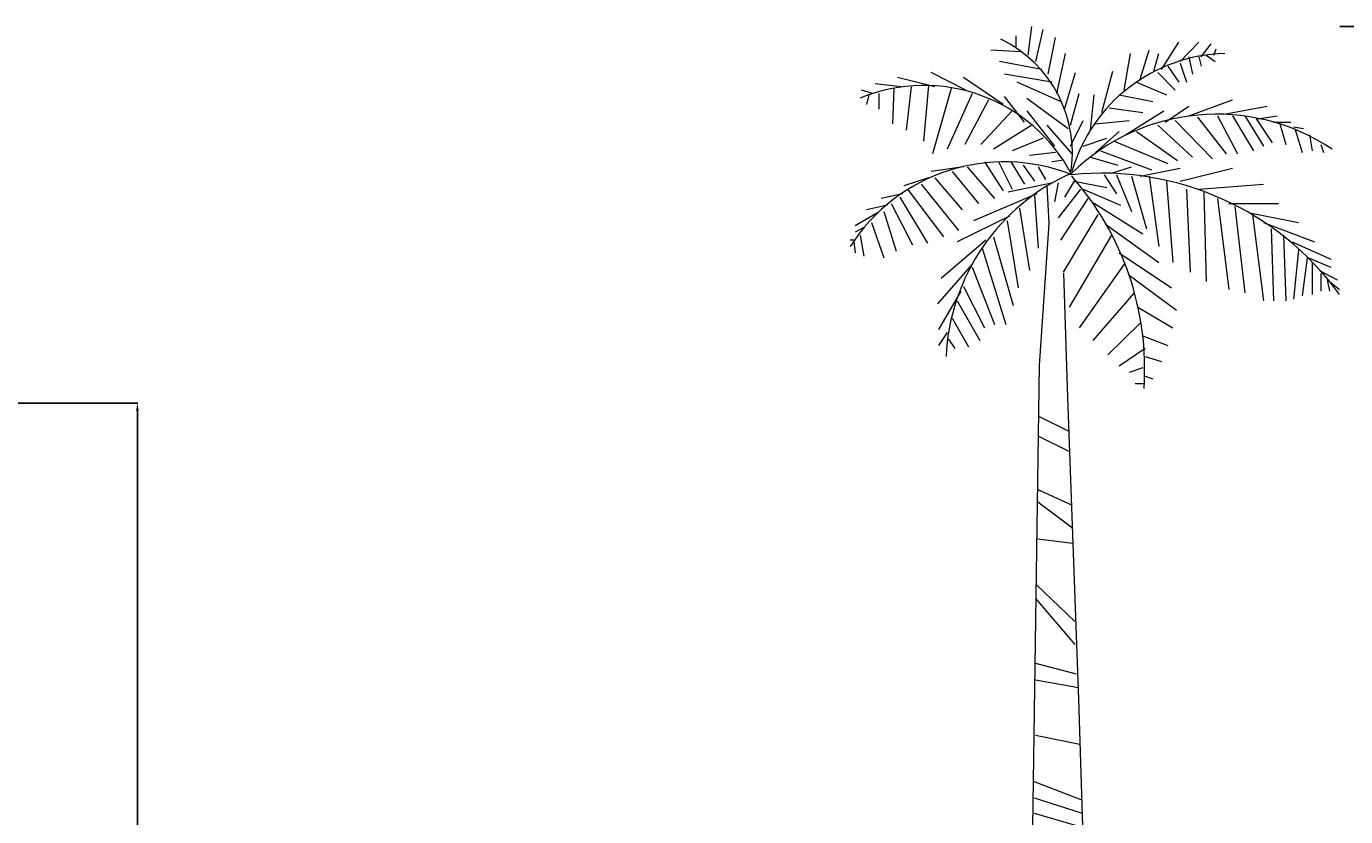
# Model space of a CAD drawing. Units: inches. Extents: x 481 to 2783, y 1975 to 3327.
# Tile 3 of 13: x 910 to 1326, y 2282 to 2531. Entities that reach past the tile are written whole.
import ezdxf

# ---------------------------------------------------------------- set-up
doc = ezdxf.new("R2010")
doc.units = ezdxf.units.IN
doc.header["$MEASUREMENT"] = 0
doc.layers.add('A-ANNO-DIMS', color=50, linetype='Continuous', lineweight=18)
doc.layers.add('L-PLNT', color=7, linetype='Continuous', lineweight=13)
doc.styles.get("Standard").update_dxf_attribs({"font": 'arial.ttf'})
doc.dimstyles.get("Standard").update_dxf_attribs({"dimtxt": 2.5, "dimasz": 2.5, "dimexe": 0.18, "dimexo": 0.0625, "dimgap": 0.09, "dimtad": 0, "dimtih": 1, "dimtoh": 1, "dimzin": 0, "dimdsep": 46, "dimlunit": 3, "dimtxsty": 'Standard', "dimcen": 0.09, "dimadec": 0, "dimazin": 0, "dimtfac": 1, "dimtofl": 0, "dimtmove": 0, "dimatfit": 3, "dimfxl": 1, "dimtolj": 1, "dimtzin": 0, "dimarcsym": 0})

# ---------------------------------------------------------------- blocks, each defined once
blk = doc.blocks.new('Tree - palm elevation')
for p, q in [((-5.567, 196.707), (-4.987, 201.167)), ((-7.5, 199.68), (-7.5, 197.946)), ((-4.407, 195.716), (-3.247, 200.672)), ((-2.474, 193.733), (-1.315, 199.433)), ((15.116, 194.477), (17.822, 198.689)), ((18.015, 195.716), (20.914, 198.689)), ((-6.727, 197.202), (-11.366, 197.45)), ((-1.121, 190.759), (0.232, 196.955)), ((9.317, 191.255), (10.283, 196.955)), ((11.829, 192.99), (13.182, 197.45)), ((13.956, 194.229), (14.729, 196.955)), ((21.301, 196.459), (22.847, 198.441)), ((22.074, 196.707), (23.427, 195.716)), ((23.234, 196.707), (23.62, 197.698)), ((-3.441, 194.477), (-10.013, 195.716)), ((16.082, 194.972), (17.822, 192.494)), ((18.015, 195.468), (18.981, 192.494)), ((19.368, 196.459), (19.948, 193.733)), ((20.914, 196.459), (21.301, 194.972)), ((-20.064, 191.751), (-25.863, 193.238)), ((-15.232, 191.255), (-20.644, 193.981)), ((-9.433, 189.025), (-15.618, 193.238)), ((-1.894, 192.494), (-9.24, 193.733)), ((0.038, 188.281), (1.778, 193.981)), ((5.837, 187.786), (7.577, 194.229)), ((14.536, 193.981), (17.242, 191.255)), ((-29.729, 190.759), (-31.469, 191.255)), ((-30.309, 190.512), (-30.695, 189.025)), ((-25.283, 191.751), (-29.342, 192.246)), ((-28.763, 190.759), (-28.763, 188.281)), ((-26.443, 191.503), (-26.636, 186.051)), ((-23.737, 191.751), (-24.51, 185.06)), ((-21.031, 191.998), (-21.804, 183.325)), ((-17.551, 191.503), (-20.451, 181.343)), ((-14.265, 190.759), (-18.131, 182.086)), ((-0.541, 189.52), (-7.307, 192.494)), ((1.005, 185.803), (2.358, 190.759)), ((4.098, 185.06), (4.678, 190.512)), ((8.544, 190.512), (13.763, 189.52)), ((11.25, 192.494), (15.889, 190.512)), ((-11.753, 189.768), (-15.425, 182.83)), ((-6.147, 186.299), (-9.24, 190.264)), ((-5.76, 190.016), (0.618, 185.308)), ((6.997, 188.529), (12.216, 187.786)), ((15.695, 186.299), (19.368, 188.777)), ((19.368, 187.29), (26.133, 189.768)), ((24.78, 187.538), (31.546, 188.777)), ((-8.08, 188.034), (-12.912, 182.83)), ((-5.76, 188.034), (-1.508, 182.582)), ((1.005, 182.582), (2.938, 186.547)), ((4.871, 186.051), (10.09, 186.547)), ((9.51, 184.317), (15.502, 188.034)), ((17.242, 186.547), (23.041, 180.599)), ((20.721, 187.042), (25.167, 181.343)), ((23.814, 187.29), (26.907, 181.343)), ((26.133, 187.29), (29.419, 181.838)), ((28.066, 187.29), (30.966, 182.582)), ((29.806, 186.795), (32.319, 183.078)), ((29.999, 186.795), (33.092, 187.29)), ((-4.987, 185.803), (-10.979, 182.086)), ((-2.668, 185.803), (1.198, 181.343)), ((4.871, 181.591), (8.544, 184.812)), ((11.25, 184.812), (17.628, 180.352)), ((14.536, 185.803), (19.948, 180.847)), ((32.512, 186.299), (35.218, 186.299)), ((33.479, 186.051), (34.445, 182.83)), ((35.605, 185.556), (37.151, 185.308)), ((35.798, 185.308), (36.958, 181.591)), ((38.118, 184.317), (38.504, 181.838)), ((-3.247, 183.821), (-8.08, 181.838)), ((2.938, 182.582), (6.61, 183.821)), ((7.77, 183.325), (16.082, 179.856)), ((39.857, 182.83), (40.244, 181.591)), ((-1.315, 181.591), (-5.374, 181.095)), ((-0.348, 180.352), (-1.894, 180.104)), ((4.098, 180.847), (8.35, 179.608)), ((5.644, 181.838), (13.569, 178.865)), ((-15.618, 179.36), (-20.644, 178.617)), ((-17.358, 178.617), (-13.299, 173.661)), ((-15.038, 179.36), (-10.786, 174.404)), ((-12.332, 180.104), (-9.433, 175.643)), ((-10.206, 180.104), (-8.08, 175.891)), ((-8.273, 180.104), (-6.147, 176.635)), ((-6.34, 179.608), (-4.6, 177.13)), ((-4.021, 179.36), (-2.861, 177.378)), ((7.384, 178.369), (10.476, 179.36)), ((11.829, 177.874), (18.015, 179.113)), ((18.015, 177.13), (26.133, 179.113)), ((-21.031, 177.626), (-24.897, 176.387)), ((-22.191, 176.635), (-16.391, 169.448)), ((-20.064, 177.626), (-15.812, 172.67)), ((-1.701, 176.882), (-8.66, 175.396)), ((-2.668, 176.387), (-2.376, 170.594)), ((-0.928, 176.882), (-1.508, 173.909)), ((1.585, 177.13), (0.038, 174.652)), ((1.585, 177.13), (6.61, 176.139)), ((6.224, 178.121), (8.157, 175.148)), ((8.157, 178.121), (10.476, 172.422)), ((10.476, 177.874), (12.796, 169.696)), ((13.182, 177.874), (14.729, 166.97)), ((15.889, 177.13), (16.855, 164.492)), ((20.914, 175.891), (30.966, 176.635)), ((-25.09, 175.148), (-28.376, 174.404)), ((-25.476, 174.652), (-21.224, 167.466)), ((-24.317, 175.891), (-18.711, 168.457)), ((-4.214, 175.148), (-14.072, 170.935)), ((-4.6, 174.9), (-4.021, 166.722)), ((2.551, 175.891), (-0.928, 171.431)), ((3.711, 174.404), (-0.541, 167.961)), ((2.938, 175.891), (8.737, 173.413)), ((18.981, 175.891), (19.561, 163.005)), ((21.688, 175.396), (22.074, 161.518)), ((23.814, 174.404), (25.554, 160.279)), ((-28.956, 172.174), (-32.435, 170.192)), ((-27.409, 173.413), (-30.695, 172.67)), ((-27.989, 172.422), (-26.056, 166.227)), ((-26.829, 173.661), (-23.544, 167.218)), ((-6.92, 172.917), (-5.374, 163.253)), ((4.291, 173.909), (12.216, 168.953)), ((25.554, 173.661), (33.285, 173.661)), ((26.52, 173.165), (28.066, 159.784)), ((28.839, 172.174), (36.378, 170.687)), ((-29.922, 170.687), (-27.989, 165.235)), ((-8.466, 171.678), (-16.585, 167.713)), ((-8.853, 170.935), (-7.113, 160.527)), ((5.257, 171.926), (-0.155, 163.005)), ((6.417, 170.439), (14.729, 164.492)), ((29.226, 171.926), (30.966, 158.545)), ((30.966, 170.687), (38.891, 167.713)), ((-32.628, 167.961), (-33.208, 167.961)), ((-31.082, 169.944), (-32.435, 169.2)), ((-31.662, 168.705), (-31.082, 165.483)), ((-12.139, 167.961), (-19.098, 162.014)), ((-10.979, 168.457), (-7.887, 157.801)), ((7.384, 168.705), (0.812, 157.553)), ((32.126, 169.696), (32.512, 158.545)), ((34.058, 168.705), (34.445, 158.545)), ((-32.628, 167.713), (-32.435, 165.979)), ((-12.719, 166.722), (-9.046, 154.828)), ((8.544, 165.979), (16.662, 160.527)), ((35.412, 167.713), (41.404, 164.988)), ((36.378, 166.474), (35.605, 158.792)), ((-14.265, 164.244), (-19.678, 158.049)), ((9.317, 164.244), (2.358, 154.332)), ((37.731, 165.235), (36.958, 159.288)), ((37.924, 165.235), (41.404, 163.749)), ((38.504, 164.492), (38.504, 159.536)), ((-14.265, 163.749), (-10.786, 154.828)), ((10.09, 162.51), (17.435, 157.058)), ((39.664, 163.253), (42.37, 161.766)), ((39.857, 162.757), (39.857, 160.031)), ((-16.005, 160.031), (-19.484, 154.084)), ((-15.618, 160.775), (-12.332, 154.332)), ((10.863, 159.784), (4.484, 152.35)), ((40.824, 161.766), (41.21, 160.031)), ((41.21, 161.518), (42.757, 160.279)), ((-16.585, 158.545), (-13.106, 152.35)), ((-17.358, 155.819), (-14.845, 151.358)), ((11.443, 157.553), (16.855, 154.332)), ((11.829, 155.075), (6.804, 150.119)), ((-18.131, 153.589), (-19.484, 151.606)), ((-17.938, 152.597), (-16.972, 151.111)), ((12.216, 153.093), (16.082, 151.606)), ((12.603, 151.111), (8.544, 148.385)), ((12.603, 149.872), (15.116, 149.128)), ((12.216, 148.137), (10.09, 147.393)), ((12.409, 145.659), (11.056, 145.659)), ((12.409, 146.898), (13.763, 146.402)), ((-4.081, 140.645), (0.753, 138.261)), ((-4.081, 137.547), (0.753, 135.163)), ((-4.081, 129.205), (1.124, 126.821)), ((-4.081, 127.298), (1.31, 123.246)), ((-4.081, 121.578), (1.31, 120.863)), ((-4.267, 114.428), (1.682, 108.708)), ((-4.453, 112.283), (1.682, 105.133)), ((-4.639, 102.273), (1.868, 100.604)), ((-4.453, 99.651), (2.24, 98.459)), ((-4.453, 91.071), (2.426, 89.641)), ((-4.825, 83.921), (2.612, 81.061)), ((-4.639, 81.299), (2.797, 78.916)), ((-4.639, 78.916), (2.797, 76.771))]:
    blk.add_line(p, q)
for points in [[(-2.363, 170.553), (-3.88, 148.505), (-4.988, 69.634), (-3.325, 24.869), (0, 0)], [(-0.116, 162.848), (0.554, 143.532), (2.217, 96.635), (3.88, 44.054), (7.76, 12.079), (11.64, 0)]]:
    blk.add_lwpolyline(points)
for centre, radius, start, end in [((-18.427, 181.448), 19.715, 350.285, 64.11229), ((25.595, 171.567), 25.395, 91.40319, 163.882), ((-21.738, 166.094), 25.899, 27.67115, 112.5305), ((23.687, 155.341), 32.188, 56.19272, 134.3213), ((-9.259, 151.732), 28.386, 68.38311, 147.5322), ((14.394, 148.393), 32.752, 113.7592, 177.4133), ((5.828, 132.718), 45.639, 35.98777, 95.82273), ((-32.8, 147.923), 45.309, 356.1943, 41.37848)]:
    blk.add_arc(centre, radius, start, end)
blk = doc.blocks.new('*D54')
at = {"layer": 'A-ANNO-DIMS', "color": 0, "lineweight": -2, "transparency": 16777216}
for p, q in [((1324.1, 2531.22), (1385.48, 2531.22)), ((1385.3, 2528.72), (1385.3, 2328.4)), ((1385.3, 2125.32), (1385.3, 2325.64)), ((1324.1, 2122.82), (1385.48, 2122.82))]:
    blk.add_line(p, q, dxfattribs=at)
at = {"layer": 'A-ANNO-DIMS', "color": 0, "transparency": 16777216}
for points in [[(1384.88, 2528.72), (1385.72, 2528.72), (1385.3, 2531.22)], [(1384.88, 2125.32), (1385.72, 2125.32), (1385.3, 2122.82)]]:
    blk.add_solid(points, dxfattribs=at)
at = {"layer": 'Defpoints', "color": 0, "transparency": 16777216}
for p in [(1324.04, 2531.22), (1385.3, 2531.22), (1324.04, 2122.82)]:
    blk.add_point(p, dxfattribs=at)
at = {"layer": 'A-ANNO-DIMS', "color": 0, "transparency": 16777216, "insert": (1385.3, 2327.02), "char_height": 2.5, "attachment_point": 5}
blk.add_mtext('\\A1;PALM 34\'-0 1/2"', dxfattribs=at)
blk = doc.blocks.new('*D58')
at = {"layer": 'A-ANNO-DIMS', "color": 0, "lineweight": -2, "transparency": 16777216}
for p, q in [((901.81, 2412.41), (945.37, 2412.41)), ((945.19, 2409.91), (945.19, 2269)), ((945.19, 2125.32), (945.19, 2266.23)), ((901.81, 2122.82), (945.37, 2122.82))]:
    blk.add_line(p, q, dxfattribs=at)
at = {"layer": 'A-ANNO-DIMS', "color": 0, "transparency": 16777216}
for points in [[(944.77, 2409.91), (945.61, 2409.91), (945.19, 2412.41)], [(944.77, 2125.32), (945.61, 2125.32), (945.19, 2122.82)]]:
    blk.add_solid(points, dxfattribs=at)
at = {"layer": 'Defpoints', "color": 0, "transparency": 16777216}
for p in [(901.75, 2412.41), (945.19, 2412.41), (901.75, 2122.82)]:
    blk.add_point(p, dxfattribs=at)
at = {"layer": 'A-ANNO-DIMS', "color": 0, "transparency": 16777216, "insert": (945.19, 2267.62), "char_height": 2.5, "attachment_point": 5}
blk.add_mtext('\\A1;EVERGREEN 24\'-1 1/2"', dxfattribs=at)

msp = doc.modelspace()

# ---------------------------------------------------------------- block references
at = {"layer": 'L-PLNT', "xscale": 2.030135039985482, "yscale": 2.030135039985482, "zscale": 2.030135039985482}
msp.add_blockref('Tree - palm elevation', (1237.239, 2122.821), dxfattribs=at)

# ---------------------------------------------------------------- dimensions: what is measured, and where the dimension line sits
at = {"layer": 'A-ANNO-DIMS'}
for base, p1, p2, text, picture, middle in [((1385.301, 2531.217), (1324.042, 2122.821), (1324.042, 2531.217), 'PALM <>', '*D54', (1385.301, 2327.019)), ((945.19, 2412.413), (901.751, 2122.821), (901.751, 2412.413), 'EVERGREEN <>', '*D58', (945.19, 2267.617))]:
    dim = msp.add_linear_dim(base=base, p1=p1, p2=p2, angle=90, text=text, dimstyle='Standard', override={"dimdec": 1, "dimlfac": 1, "dimrnd": 0, "dimzin": 1, "dimdsep": 46, "dimlunit": 4, "dimfrac": 2}, dxfattribs=at)
    dim.commit()
    dim.dimension.update_dxf_attribs({"geometry": picture, "text_midpoint": middle})

doc.saveas('drawing.dxf')
